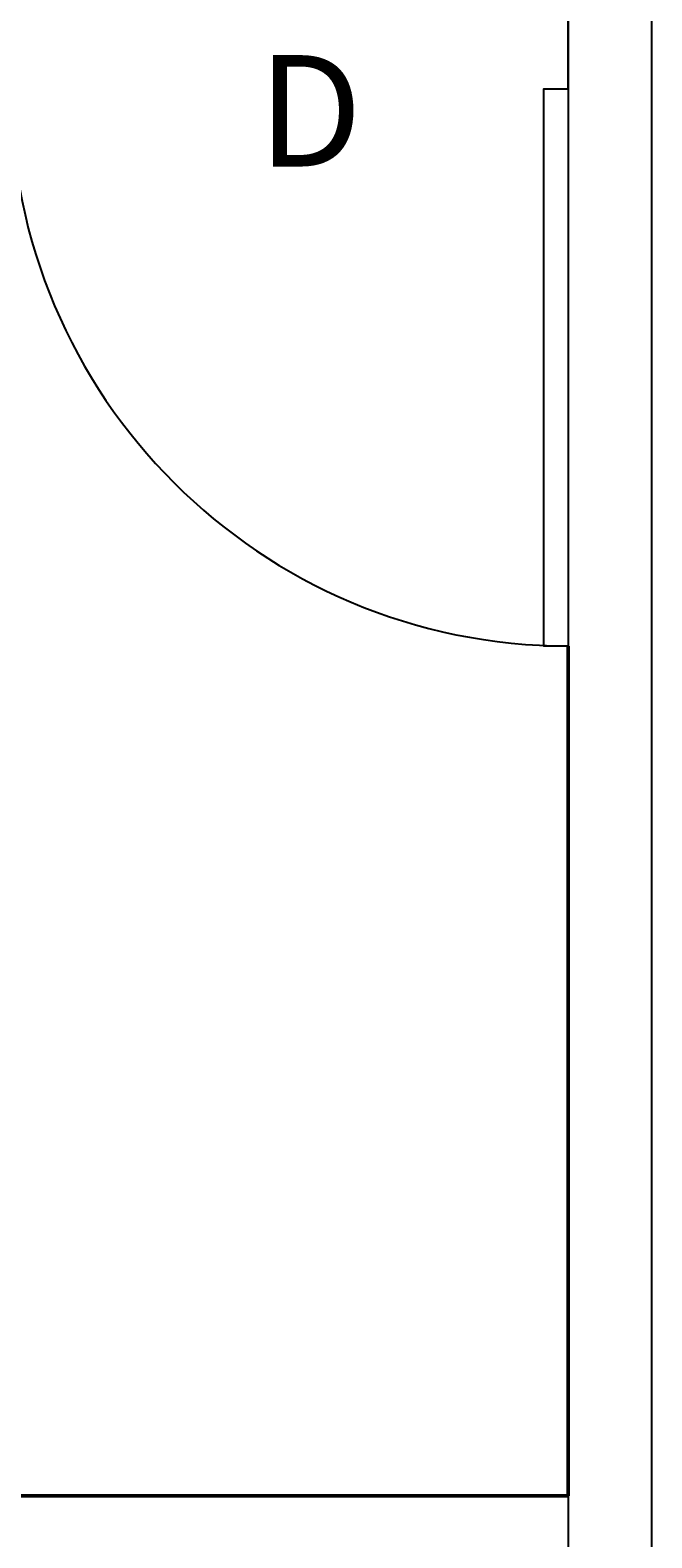
# Model space of a CAD drawing. Units: inches. Extents: x 37 to 824, y -700 to 234.
# Tile 35 of 77: x 251 to 296, y -269 to -161. Entities that reach past the tile are written whole.
import ezdxf

# ---------------------------------------------------------------- set-up
doc = ezdxf.new("R2010")
doc.units = ezdxf.units.IN
doc.header["$MEASUREMENT"] = 0
for name, color, linetype, lineweight in [('A-ANNO-DIMS', 2, 'Continuous', 18), ('A-ANNO-TEXT', 7, 'Continuous', 18), ('A-DOOR', 4, 'Continuous', 25), ('A-WALL', 2, 'Continuous', 50)]:
    doc.layers.add(name, color=color, linetype=linetype, lineweight=lineweight)
doc.styles.get("Standard").update_dxf_attribs({"font": 'arial.ttf'})
doc.dimstyles.get("Standard").update_dxf_attribs({"dimtxt": 0.18, "dimasz": 0.18, "dimexe": 0.18, "dimexo": 0.0625, "dimgap": 0.09, "dimtad": 0, "dimtih": 1, "dimtoh": 1, "dimdec": 1, "dimzin": 0, "dimdsep": 46, "dimlunit": 4, "dimtxsty": 'Standard', "dimcen": 0.09, "dimadec": 0, "dimazin": 0, "dimtfac": 1, "dimtdec": 1, "dimtofl": 0, "dimtmove": 0, "dimatfit": 3, "dimfxl": 1, "dimtolj": 1, "dimtzin": 0, "dimarcsym": 0})

# ---------------------------------------------------------------- blocks, each defined once
blk = doc.blocks.new('*U2')
for p, q in [((-40, 0), (-40, 6)), ((0, 0), (0, 6))]:
    blk.add_line(p, q)
blk.add_lwpolyline([(0, 0), (0, -40), (-1.75, -40), (-1.75, 0)], close=True)
blk.add_arc((0, 0), 40, 180, 270)
blk = doc.blocks.new('*D77')
at = {"layer": 'A-ANNO-DIMS', "color": 0, "lineweight": -2, "ltscale": 0.5, "transparency": 16777216}
for p, q in [((227.08, 45.5), (227.08, -400.41)), ((290.08, 15.03), (290.08, -400.41)), ((227.26, -400.23), (258.25, -400.23)), ((289.9, -400.23), (258.91, -400.23))]:
    blk.add_line(p, q, dxfattribs=at)
at = {"layer": 'A-ANNO-DIMS', "color": 0, "ltscale": 0.5, "transparency": 16777216}
for points in [[(227.26, -400.2), (227.26, -400.26), (227.08, -400.23)], [(289.9, -400.2), (289.9, -400.26), (290.08, -400.23)]]:
    blk.add_solid(points, dxfattribs=at)
at = {"layer": 'Defpoints', "color": 0, "ltscale": 0.5, "transparency": 16777216}
for p in [(227.08, 45.56), (290.08, 15.09), (290.08, -400.23)]:
    blk.add_point(p, dxfattribs=at)
at = {"layer": 'A-ANNO-DIMS', "color": 0, "ltscale": 0.5, "transparency": 16777216, "insert": (258.58, -400.23), "char_height": 0.18, "attachment_point": 5}
blk.add_mtext('\\A1;5\'-3"', dxfattribs=at)
blk = doc.blocks.new('*D81')
at = {"layer": 'A-ANNO-DIMS', "color": 0, "lineweight": -2, "ltscale": 0.5, "transparency": 16777216}
for p, q in [((290.08, -164.97), (290.08, -400.41)), ((250.19, -167.97), (250.19, -400.41)), ((250.37, -400.23), (269.8, -400.23)), ((289.9, -400.23), (270.46, -400.23))]:
    blk.add_line(p, q, dxfattribs=at)
at = {"layer": 'A-ANNO-DIMS', "color": 0, "ltscale": 0.5, "transparency": 16777216}
for points in [[(250.37, -400.2), (250.37, -400.26), (250.19, -400.23)], [(289.9, -400.2), (289.9, -400.26), (290.08, -400.23)]]:
    blk.add_solid(points, dxfattribs=at)
at = {"layer": 'Defpoints', "color": 0, "ltscale": 0.5, "transparency": 16777216}
for p in [(290.08, -164.91), (250.19, -167.91), (290.08, -400.23)]:
    blk.add_point(p, dxfattribs=at)
at = {"layer": 'A-ANNO-DIMS', "color": 0, "ltscale": 0.5, "transparency": 16777216, "insert": (270.13, -400.23), "char_height": 0.18, "attachment_point": 5}
blk.add_mtext('\\A1;3\'-4"', dxfattribs=at)
blk = doc.blocks.new('*D87')
at = {"layer": 'A-ANNO-DIMS', "color": 0, "lineweight": -2, "ltscale": 0.5, "transparency": 16777216}
for p, q in [((216.08, -356.85), (216.08, 234.17)), ((216.26, 233.99), (255.75, 233.99)), ((295.9, 233.99), (256.41, 233.99)), ((296.08, -356.85), (296.08, 234.17))]:
    blk.add_line(p, q, dxfattribs=at)
at = {"layer": 'A-ANNO-DIMS', "color": 0, "ltscale": 0.5, "transparency": 16777216}
for points in [[(216.26, 234.02), (216.26, 233.96), (216.08, 233.99)], [(295.9, 234.02), (295.9, 233.96), (296.08, 233.99)]]:
    blk.add_solid(points, dxfattribs=at)
at = {"layer": 'Defpoints', "color": 0, "ltscale": 0.5, "transparency": 16777216}
for p in [(296.08, 233.99), (216.08, -356.91), (296.08, -356.91)]:
    blk.add_point(p, dxfattribs=at)
at = {"layer": 'A-ANNO-DIMS', "color": 0, "ltscale": 0.5, "transparency": 16777216, "insert": (256.08, 233.99), "char_height": 0.18, "attachment_point": 5}
blk.add_mtext('\\A1;6\'-8"', dxfattribs=at)

msp = doc.modelspace()

# ---------------------------------------------------------------- linework, layer by layer
at = {"layer": 'A-WALL'}
for p, q in [((290.08, -206.91), (290.08, -204.91)), ((290.08, -204.91), (290.08, -265.91)), ((290.08, -265.91), (290.08, -215.91)), ((290.08, -265.91), (170.08, -265.91))]:
    msp.add_line(p, q, dxfattribs=at)

# ---------------------------------------------------------------- block references
at = {"layer": 'A-DOOR'}
msp.add_blockref('*U2', (290.08, -164.91), dxfattribs=at)

# ---------------------------------------------------------------- texts
at = {"layer": 'A-ANNO-TEXT'}
msp.add_text('D', height=8, dxfattribs=at).set_placement((267.8, -170.49))

# ---------------------------------------------------------------- dimensions: what is measured, and where the dimension line sits
at = {"layer": 'A-ANNO-DIMS', "ltscale": 0.5}
for base, p1, p2, picture, middle in [((296.08, 233.99), (216.08, -356.91), (296.08, -356.91), '*D87', (256.08, 233.99)), ((290.08, -400.23), (227.08, 45.56), (290.08, 15.09), '*D77', (258.58, -400.23)), ((290.08, -400.23), (250.19, -167.91), (290.08, -164.91), '*D81', (270.13, -400.23))]:
    dim = msp.add_linear_dim(base=base, p1=p1, p2=p2, dimstyle='Standard', override={"dimdec": 1, "dimlfac": 1, "dimrnd": 0, "dimzin": 1, "dimdsep": 46, "dimlunit": 4, "dimfrac": 2}, dxfattribs=at)
    dim.commit()
    dim.dimension.update_dxf_attribs({"geometry": picture, "text_midpoint": middle})

doc.saveas('drawing.dxf')
